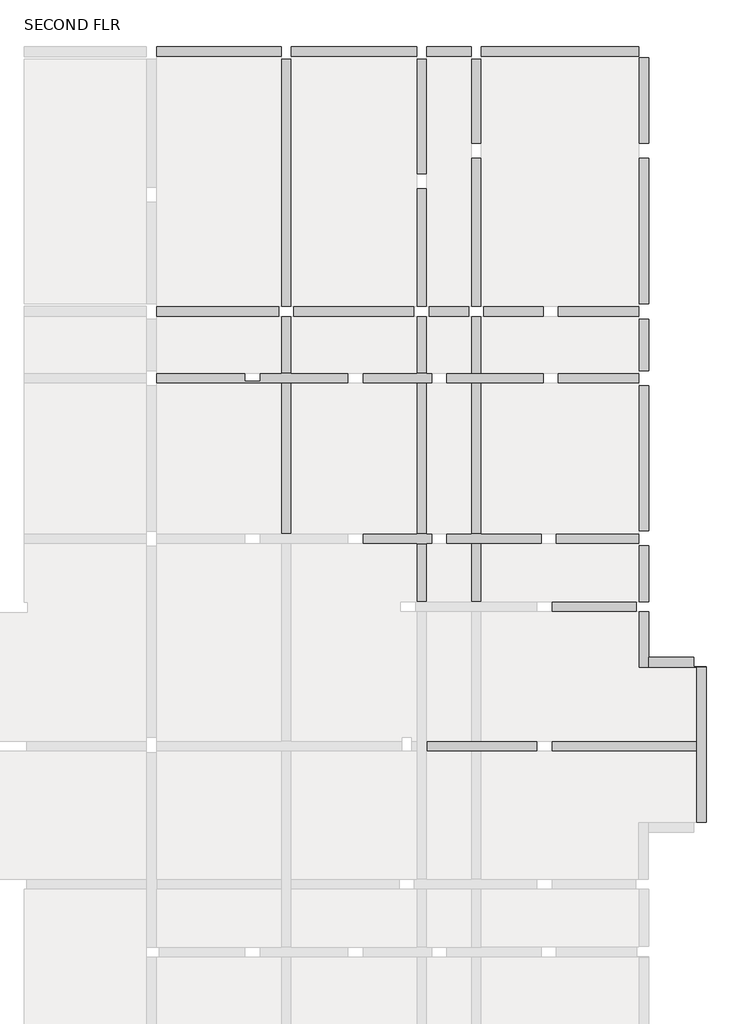
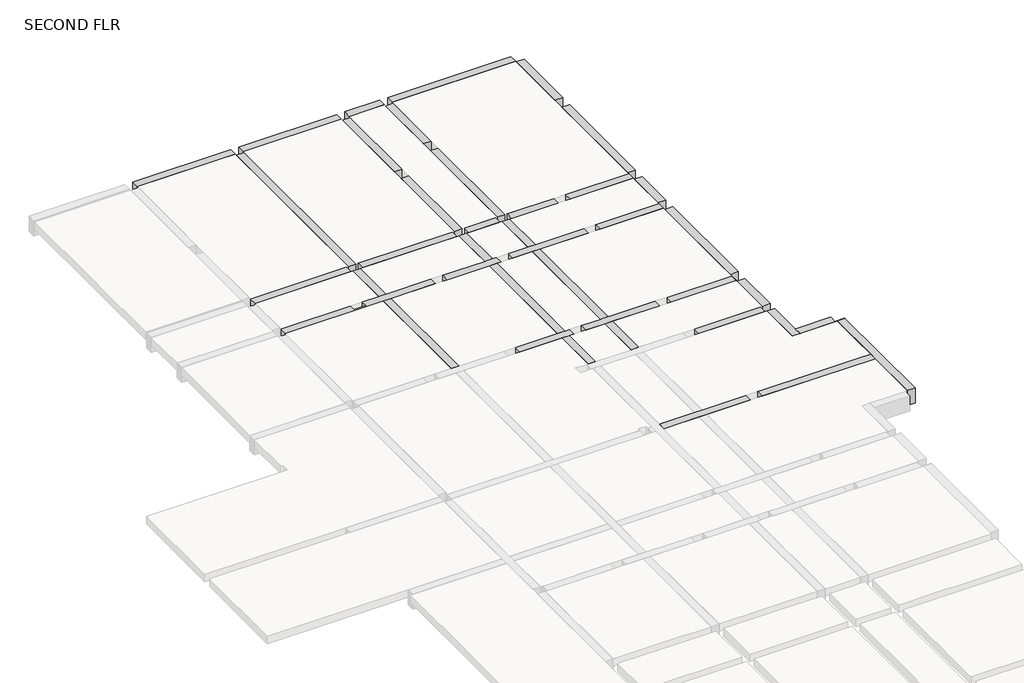
# One storey, part 4 of 4: 40 beams.
"""IFC4 building model written with IfcOpenShell, lengths in millimetres."""

from ifc_helpers import new_model, si_unit, frame, origin, place, context, project, spatial, polyline, outline, extrude, faceted_brep, element, save

model = new_model("IFC4")

# Units and contexts
model_context = context("Model", 3, world=origin())
ifc_project = project(units=[si_unit("LENGTHUNIT", "METRE", prefix="MILLI")], contexts=[model_context])

# Site, building, storey
site = spatial("IfcSite", under=ifc_project)
building = spatial("IfcBuilding", under=site)
storey = spatial("IfcBuildingStorey", under=building, Name="SECOND FLR", Elevation=6048.0)

# Beams
placement = place(None, origin())
element("IfcBeam", 1, ObjectType="M_Concrete-Rectangular Beam : 300 x 600mm", at=placement, inside=storey, context=model_context, shape_type="Brep", body=[
    faceted_brep([(2024.7296816, 21537.8349362, 6048.0), (2024.7296816, 21837.8349362, 6048.0), (-1671.7865686, 21837.8349362, 6048.0), (-1671.7865686, 21537.8349362, 6048.0), (2024.7296816, 21537.8349362, 5448.0), (2024.7296816, 21537.8349362, 5748.0), (-1671.7865686, 21537.8349362, 5748.0), (-1671.7865686, 21537.8349362, 5448.0), (2024.7296816, 21837.8349362, 5448.0), (-1671.7865686, 21837.8349362, 5448.0)], [[[0, 1, 2, 3]], [[4, 5, 0, 3, 6, 7]], [[8, 4, 7, 9]], [[1, 8, 9, 2]], [[2, 9, 7, 6, 3]], [[1, 0, 5, 4, 8]]]),
])
element("IfcBeam", 2, ObjectType="M_Concrete-Rectangular Beam : 300 x 600mm", at=placement, inside=storey, context=model_context, shape_type="Brep", body=[
    faceted_brep([(6032.5248054, 21537.8349362, 6048.0), (6032.5248054, 21837.8349362, 6048.0), (2324.7296816, 21837.8349362, 6048.0), (2324.7296816, 21537.8349362, 6048.0), (6032.5248054, 21537.8349362, 5448.0), (6032.5248054, 21537.8349362, 5748.0), (2324.7296816, 21537.8349362, 5748.0), (2324.7296816, 21537.8349362, 5448.0), (6032.5248054, 21837.8349362, 5448.0), (2324.7296816, 21837.8349362, 5448.0)], [[[0, 1, 2, 3]], [[4, 5, 0, 3, 6, 7]], [[8, 4, 7, 9]], [[1, 8, 9, 2]], [[2, 9, 7, 6, 3]], [[1, 0, 5, 4, 8]]]),
])
element("IfcBeam", 3, ObjectType="M_Concrete-Rectangular Beam : 300 x 600mm", at=placement, inside=storey, context=model_context, shape_type="Brep", body=[
    faceted_brep([(7656.8679014, 21537.8349362, 6048.0), (7656.8679014, 21837.8349362, 6048.0), (6332.5248054, 21837.8349362, 6048.0), (6332.5248054, 21537.8349362, 6048.0), (7656.8679014, 21537.8349362, 5448.0), (7656.8679014, 21537.8349362, 5748.0), (6332.5248054, 21537.8349362, 5748.0), (6332.5248054, 21537.8349362, 5448.0), (7656.8679014, 21837.8349362, 5448.0), (6332.5248054, 21837.8349362, 5448.0)], [[[0, 1, 2, 3]], [[4, 5, 0, 3, 6, 7]], [[8, 4, 7, 9]], [[1, 8, 9, 2]], [[2, 9, 7, 6, 3]], [[1, 0, 5, 4, 8]]]),
])
element("IfcBeam", 4, ObjectType="M_Concrete-Rectangular Beam : 300 x 600mm", at=placement, inside=storey, context=model_context, shape_type="Brep", body=[
    faceted_brep([(7956.8679014, 21837.8349362, 6048.0), (7956.8679014, 21537.8349362, 6048.0), (12619.1163908, 21537.8349362, 6048.0), (12619.1163908, 21837.8349362, 6048.0), (7956.8679014, 21537.8349362, 5748.0), (7956.8679014, 21537.8349362, 5448.0), (12619.1163908, 21537.8349362, 5448.0), (12619.1163908, 21537.8349362, 5748.0), (7956.8679014, 21837.8349362, 5448.0), (12619.1163908, 21837.8349362, 5448.0)], [[[0, 1, 2, 3]], [[1, 4, 5, 6, 7, 2]], [[5, 8, 9, 6]], [[8, 0, 3, 9]], [[0, 8, 5, 4, 1]], [[3, 2, 7, 6, 9]]]),
])
element("IfcBeam", 5, ObjectType="M_Concrete-Rectangular Beam : 300 x 600mm", at=placement, inside=storey, context=model_context, shape_type="Brep", body=[
    faceted_brep([(14319.1163908, 3443.0536525, 6048.0), (14619.1163908, 3443.0536525, 6048.0), (14619.1163908, 3443.0536525, 5448.0), (14319.1163908, 3443.0536525, 5448.0), (14319.1163908, 3435.7536525, 6048.0), (14319.1163908, 1251.1713929, 6048.0), (14319.1163908, 951.1713929, 6048.0), (14319.1163908, -1148.8286071, 6048.0), (14619.1163908, -1148.8286071, 6048.0), (14619.1163908, -1148.8286071, 5448.0), (14319.1163908, -1148.8286071, 5448.0), (14319.1163908, 951.1713929, 5448.0), (14319.1163908, 1251.1713929, 5448.0), (14319.1163908, 3435.7536525, 5448.0), (14319.1163908, -1148.8286071, 5748.0)], [[[0, 1, 2, 3]], [[1, 0, 4, 5, 6, 7, 8]], [[2, 1, 8, 9]], [[3, 2, 9, 10, 11, 12, 13]], [[0, 3, 13, 12, 11, 10, 14, 7, 6, 5, 4]], [[7, 14, 10, 9, 8]]]),
])
element("IfcBeam", 6, ObjectType="M_Concrete-Rectangular Beam : 300 x 600mm", at=placement, inside=storey, context=model_context, shape_type="Brep", body=[
    faceted_brep([(12916.8679014, 5087.6057249, 6048.0), (12616.8679014, 5087.6057249, 6048.0), (12616.8679014, 3435.7536525, 6048.0), (12916.8679014, 3435.7536525, 6048.0), (12916.8679014, 3735.7536525, 6048.0), (12616.8679014, 5087.6057249, 5748.0), (12616.8679014, 5087.6057249, 5448.0), (12616.8679014, 3435.7536525, 5448.0), (12616.8679014, 3435.7536525, 5748.0), (12916.8679014, 5087.6057249, 5448.0), (12916.8679014, 3735.7536525, 5448.0), (12916.8679014, 3435.7536525, 5448.0), (12916.8679014, 3435.7536525, 5748.0)], [[[0, 1, 2, 3, 4]], [[2, 1, 5, 6, 7, 8]], [[6, 9, 10, 11, 7]], [[9, 0, 4, 3, 12, 11, 10]], [[0, 9, 6, 5, 1]], [[3, 2, 8, 7, 11, 12]]]),
])
element("IfcBeam", 7, ObjectType="M_Concrete-Rectangular Beam : 300 x 600mm", at=placement, inside=storey, context=model_context, shape_type="Brep", body=[
    faceted_brep([(12916.8679014, 3735.7536525, 6048.0), (12916.8679014, 3435.7536525, 6048.0), (14319.1163908, 3435.7536525, 6048.0), (14319.1163908, 3443.0536525, 6048.0), (14619.1163908, 3443.0536525, 6048.0), (14619.1163908, 3455.7536525, 6048.0), (14244.1163908, 3455.7536525, 6048.0), (14244.1163908, 3735.7536525, 6048.0), (12916.8679014, 3735.7536525, 5448.0), (14244.1163908, 3735.7536525, 5448.0), (12916.8679014, 3435.7536525, 5448.0), (14244.1163908, 3455.7536525, 5448.0), (14619.1163908, 3455.7536525, 5448.0), (14619.1163908, 3443.0536525, 5448.0), (14319.1163908, 3443.0536525, 5448.0), (14319.1163908, 3435.7536525, 5448.0), (12916.8679014, 3435.7536525, 5748.0), (14319.1163908, 3435.7536525, 5748.0)], [[[0, 1, 2, 3, 4, 5, 6, 7]], [[8, 0, 7, 9]], [[10, 8, 9, 11, 12, 13, 14, 15]], [[2, 1, 16, 10, 15, 17]], [[1, 0, 8, 10, 16]], [[12, 5, 4, 13]], [[7, 6, 11, 9]], [[11, 6, 5, 12]], [[3, 14, 13, 4]], [[14, 3, 2, 17, 15]]]),
])
element("IfcBeam", 8, ObjectType="M_Concrete-Rectangular Beam : 300 x 600mm", at=placement, inside=storey, context=model_context, shape_type="Brep", body=[
    faceted_brep([(12616.8679014, 5387.6057249, 6048.0), (12916.8679014, 5387.6057249, 6048.0), (12916.8679014, 7044.7076276, 6048.0), (12619.1163908, 7044.7076276, 6048.0), (12619.1163908, 7399.7076276, 6048.0), (12616.8679014, 7399.7076276, 6048.0), (12616.8679014, 7099.7076276, 6048.0), (12616.8679014, 7399.7076276, 5448.0), (12616.8679014, 7099.7076276, 5448.0), (12616.8679014, 5387.6057249, 5448.0), (12616.8679014, 5387.6057249, 5748.0), (12616.8679014, 7399.7076276, 5748.0), (12916.8679014, 5387.6057249, 5448.0), (12619.1163908, 7399.7076276, 5448.0), (12619.1163908, 7044.7076276, 5448.0), (12916.8679014, 7044.7076276, 5448.0)], [[[0, 1, 2, 3, 4, 5, 6]], [[7, 8, 9, 10, 0, 6, 5, 11]], [[12, 9, 8, 7, 13, 14, 15]], [[1, 12, 15, 2]], [[1, 0, 10, 9, 12]], [[14, 3, 2, 15]], [[3, 14, 13, 4]], [[5, 4, 13, 7, 11]]]),
])
element("IfcBeam", 9, ObjectType="M_Concrete-Rectangular Beam : 300 x 600mm", at=placement, inside=storey, context=model_context, shape_type="SweptSolid", body=[
    extrude(outline(polyline([(12619.1163908, 11782.4075451), (12919.1163908, 11782.4075451), (12919.1163908, 7494.7076276), (12619.1163908, 7494.7076276), (12619.1163908, 11782.4075451)])), frame((0.0, 0.0, 5448.0), z_axis=(0.0, 0.0, 1.0), x_axis=(1.0, 0.0, 0.0)), (0.0, 0.0, 1.0), 600.0),
])
element("IfcBeam", 10, ObjectType="M_Concrete-Rectangular Beam : 300 x 600mm", at=placement, inside=storey, context=model_context, shape_type="Brep", body=[
    faceted_brep([(12619.1163908, 13762.5179708, 6048.0), (12619.1163908, 12232.4075451, 6048.0), (12919.1163908, 12232.4075451, 6048.0), (12919.1163908, 13762.5179708, 6048.0), (12919.1163908, 12232.4075451, 5448.0), (12919.1163908, 13762.5179708, 5448.0), (12619.1163908, 12232.4075451, 5448.0), (12619.1163908, 13762.5179708, 5448.0), (12619.1163908, 13762.5179708, 5748.0), (12619.1163908, 12232.4075451, 5748.0)], [[[0, 1, 2, 3]], [[3, 2, 4, 5]], [[5, 4, 6, 7]], [[1, 0, 8, 7, 6, 9]], [[0, 3, 5, 7, 8]], [[6, 4, 2, 1, 9]]]),
])
element("IfcBeam", 11, ObjectType="M_Concrete-Rectangular Beam : 300 x 600mm", at=placement, inside=storey, context=model_context, shape_type="Brep", body=[
    faceted_brep([(12619.1163908, 18524.7148651, 6048.0), (12619.1163908, 14212.5179708, 6048.0), (12919.1163908, 14212.5179708, 6048.0), (12919.1163908, 18524.7148651, 6048.0), (12919.1163908, 14212.5179708, 5448.0), (12919.1163908, 18524.7148651, 5448.0), (12619.1163908, 14212.5179708, 5448.0), (12619.1163908, 18524.7148651, 5448.0), (12619.1163908, 18524.7148651, 5748.0), (12619.1163908, 14212.5179708, 5748.0)], [[[0, 1, 2, 3]], [[3, 2, 4, 5]], [[5, 4, 6, 7]], [[1, 0, 8, 7, 6, 9]], [[0, 3, 5, 7, 8]], [[6, 4, 2, 1, 9]]]),
])
element("IfcBeam", 12, ObjectType="M_Concrete-Rectangular Beam : 300 x 600mm", at=placement, inside=storey, context=model_context, shape_type="Brep", body=[
    faceted_brep([(12619.1163908, 21502.8349362, 6048.0), (12619.1163908, 18974.7148651, 6048.0), (12919.1163908, 18974.7148651, 6048.0), (12919.1163908, 21502.8349362, 6048.0), (12919.1163908, 18974.7148651, 5448.0), (12919.1163908, 21502.8349362, 5448.0), (12619.1163908, 18974.7148651, 5448.0), (12619.1163908, 21502.8349362, 5448.0), (12619.1163908, 21502.8349362, 5748.0), (12619.1163908, 18974.7148651, 5748.0)], [[[0, 1, 2, 3]], [[3, 2, 4, 5]], [[5, 4, 6, 7]], [[1, 0, 8, 7, 6, 9]], [[6, 4, 2, 1, 9]], [[0, 3, 5, 7, 8]]]),
])
element("IfcBeam", 13, ObjectType="M_Concrete-Rectangular Beam : 300 x 600mm", at=placement, inside=storey, context=model_context, shape_type="Brep", body=[
    faceted_brep([(2324.7296816, 21462.8349362, 6048.0), (2024.7296816, 21462.8349362, 6048.0), (2024.7296816, 14137.5179708, 6048.0), (2324.7296816, 14137.5179708, 6048.0), (2024.7296816, 21462.8349362, 5748.0), (2024.7296816, 21462.8349362, 5448.0), (2024.7296816, 14137.5179708, 5448.0), (2024.7296816, 14137.5179708, 5748.0), (2324.7296816, 21462.8349362, 5448.0), (2324.7296816, 14137.5179708, 5448.0), (2324.7296816, 14137.5179708, 5748.0), (2324.7296816, 21462.8349362, 5748.0)], [[[0, 1, 2, 3]], [[2, 1, 4, 5, 6, 7]], [[5, 8, 9, 6]], [[0, 3, 10, 9, 8, 11]], [[1, 0, 11, 8, 5, 4]], [[3, 2, 7, 6, 9, 10]]]),
])
element("IfcBeam", 14, ObjectType="M_Concrete-Rectangular Beam : 300 x 600mm", at=placement, inside=storey, context=model_context, shape_type="Brep", body=[
    faceted_brep([(2324.7296816, 13837.5179708, 6048.0), (2024.7296816, 13837.5179708, 6048.0), (2024.7296816, 12157.4075451, 6048.0), (2324.7296816, 12157.4075451, 6048.0), (2024.7296816, 13837.5179708, 5748.0), (2024.7296816, 13837.5179708, 5448.0), (2024.7296816, 12157.4075451, 5448.0), (2024.7296816, 12157.4075451, 5748.0), (2324.7296816, 13837.5179708, 5448.0), (2324.7296816, 12157.4075451, 5448.0), (2324.7296816, 12157.4075451, 5748.0), (2324.7296816, 13837.5179708, 5748.0)], [[[0, 1, 2, 3]], [[2, 1, 4, 5, 6, 7]], [[5, 8, 9, 6]], [[0, 3, 10, 9, 8, 11]], [[1, 0, 11, 8, 5, 4]], [[3, 2, 7, 6, 9, 10]]]),
])
element("IfcBeam", 15, ObjectType="M_Concrete-Rectangular Beam : 300 x 600mm", at=placement, inside=storey, context=model_context, shape_type="Brep", body=[
    faceted_brep([(6332.5248054, 21462.8349362, 6048.0), (6032.5248054, 21462.8349362, 6048.0), (6032.5248054, 18074.7148651, 6048.0), (6332.5248054, 18074.7148651, 6048.0), (6032.5248054, 21462.8349362, 5748.0), (6032.5248054, 21462.8349362, 5448.0), (6032.5248054, 18074.7148651, 5448.0), (6032.5248054, 18074.7148651, 5748.0), (6332.5248054, 21462.8349362, 5448.0), (6332.5248054, 18074.7148651, 5448.0), (6332.5248054, 18074.7148651, 5748.0), (6332.5248054, 21462.8349362, 5748.0)], [[[0, 1, 2, 3]], [[2, 1, 4, 5, 6, 7]], [[5, 8, 9, 6]], [[0, 3, 10, 9, 8, 11]], [[1, 0, 11, 8, 5, 4]], [[3, 2, 7, 6, 9, 10]]]),
])
element("IfcBeam", 16, ObjectType="M_Concrete-Rectangular Beam : 300 x 600mm", at=placement, inside=storey, context=model_context, shape_type="Brep", body=[
    faceted_brep([(6332.5248054, 17624.7148651, 6048.0), (6032.5248054, 17624.7148651, 6048.0), (6032.5248054, 14137.5179708, 6048.0), (6332.5248054, 14137.5179708, 6048.0), (6032.5248054, 17624.7148651, 5748.0), (6032.5248054, 17624.7148651, 5448.0), (6032.5248054, 14137.5179708, 5448.0), (6032.5248054, 14137.5179708, 5748.0), (6332.5248054, 17624.7148651, 5448.0), (6332.5248054, 14137.5179708, 5448.0), (6332.5248054, 14137.5179708, 5748.0), (6332.5248054, 17624.7148651, 5748.0)], [[[0, 1, 2, 3]], [[2, 1, 4, 5, 6, 7]], [[5, 8, 9, 6]], [[0, 3, 10, 9, 8, 11]], [[1, 0, 11, 8, 5, 4]], [[3, 2, 7, 6, 9, 10]]]),
])
element("IfcBeam", 17, ObjectType="M_Concrete-Rectangular Beam : 300 x 600mm", at=placement, inside=storey, context=model_context, shape_type="Brep", body=[
    faceted_brep([(6332.5248054, 13837.5179708, 6048.0), (6032.5248054, 13837.5179708, 6048.0), (6032.5248054, 12157.4075451, 6048.0), (6332.5248054, 12157.4075451, 6048.0), (6032.5248054, 13837.5179708, 5748.0), (6032.5248054, 13837.5179708, 5448.0), (6032.5248054, 12157.4075451, 5448.0), (6032.5248054, 12157.4075451, 5748.0), (6332.5248054, 13837.5179708, 5448.0), (6332.5248054, 12157.4075451, 5448.0), (6332.5248054, 12157.4075451, 5748.0), (6332.5248054, 13837.5179708, 5748.0)], [[[0, 1, 2, 3]], [[2, 1, 4, 5, 6, 7]], [[5, 8, 9, 6]], [[0, 3, 10, 9, 8, 11]], [[1, 0, 11, 8, 5, 4]], [[3, 2, 7, 6, 9, 10]]]),
])
element("IfcBeam", 18, ObjectType="M_Concrete-Rectangular Beam : 300 x 600mm", at=placement, inside=storey, context=model_context, shape_type="Brep", body=[
    faceted_brep([(7956.8679014, 21462.8349362, 6048.0), (7656.8679014, 21462.8349362, 6048.0), (7656.8679014, 18974.7148651, 6048.0), (7956.8679014, 18974.7148651, 6048.0), (7656.8679014, 21462.8349362, 5748.0), (7656.8679014, 21462.8349362, 5448.0), (7656.8679014, 18974.7148651, 5448.0), (7656.8679014, 18974.7148651, 5748.0), (7956.8679014, 21462.8349362, 5448.0), (7956.8679014, 18974.7148651, 5448.0), (7956.8679014, 18974.7148651, 5748.0), (7956.8679014, 21462.8349362, 5748.0)], [[[0, 1, 2, 3]], [[2, 1, 4, 5, 6, 7]], [[5, 8, 9, 6]], [[0, 3, 10, 9, 8, 11]], [[1, 0, 11, 8, 5, 4]], [[3, 2, 7, 6, 9, 10]]]),
])
element("IfcBeam", 19, ObjectType="M_Concrete-Rectangular Beam : 300 x 600mm", at=placement, inside=storey, context=model_context, shape_type="Brep", body=[
    faceted_brep([(7956.8679014, 18524.7148651, 6048.0), (7656.8679014, 18524.7148651, 6048.0), (7656.8679014, 14137.5179708, 6048.0), (7956.8679014, 14137.5179708, 6048.0), (7656.8679014, 18524.7148651, 5748.0), (7656.8679014, 18524.7148651, 5448.0), (7656.8679014, 14137.5179708, 5448.0), (7656.8679014, 14137.5179708, 5748.0), (7956.8679014, 18524.7148651, 5448.0), (7956.8679014, 14137.5179708, 5448.0), (7956.8679014, 14137.5179708, 5748.0), (7956.8679014, 18524.7148651, 5748.0)], [[[0, 1, 2, 3]], [[2, 1, 4, 5, 6, 7]], [[5, 8, 9, 6]], [[0, 3, 10, 9, 8, 11]], [[1, 0, 11, 8, 5, 4]], [[3, 2, 7, 6, 9, 10]]]),
])
element("IfcBeam", 20, ObjectType="M_Concrete-Rectangular Beam : 300 x 600mm", at=placement, inside=storey, context=model_context, shape_type="Brep", body=[
    faceted_brep([(7956.8679014, 13837.5179708, 6048.0), (7656.8679014, 13837.5179708, 6048.0), (7656.8679014, 12157.4075451, 6048.0), (7956.8679014, 12157.4075451, 6048.0), (7656.8679014, 13837.5179708, 5748.0), (7656.8679014, 13837.5179708, 5448.0), (7656.8679014, 12157.4075451, 5448.0), (7656.8679014, 12157.4075451, 5748.0), (7956.8679014, 13837.5179708, 5448.0), (7956.8679014, 12157.4075451, 5448.0), (7956.8679014, 12157.4075451, 5748.0), (7956.8679014, 13837.5179708, 5748.0)], [[[0, 1, 2, 3]], [[2, 1, 4, 5, 6, 7]], [[5, 8, 9, 6]], [[0, 3, 10, 9, 8, 11]], [[1, 0, 11, 8, 5, 4]], [[3, 2, 7, 6, 9, 10]]]),
])
element("IfcBeam", 21, ObjectType="M_Concrete-Rectangular Beam : 300 x 600mm", at=placement, inside=storey, context=model_context, shape_type="Brep", body=[
    faceted_brep([(-1671.7865686, 14137.5179708, 6048.0), (-1671.7865686, 13837.5179708, 6048.0), (1949.7296816, 13837.5179708, 6048.0), (1949.7296816, 14137.5179708, 6048.0), (-1671.7865686, 13837.5179708, 5748.0), (-1671.7865686, 13837.5179708, 5448.0), (1949.7296816, 13837.5179708, 5448.0), (1949.7296816, 13837.5179708, 5748.0), (-1671.7865686, 14137.5179708, 5448.0), (1949.7296816, 14137.5179708, 5448.0), (1949.7296816, 14137.5179708, 5748.0), (-1671.7865686, 14137.5179708, 5748.0)], [[[0, 1, 2, 3]], [[2, 1, 4, 5, 6, 7]], [[5, 8, 9, 6]], [[0, 3, 10, 9, 8, 11]], [[1, 0, 11, 8, 5, 4]], [[3, 2, 7, 6, 9, 10]]]),
])
element("IfcBeam", 22, ObjectType="M_Concrete-Rectangular Beam : 300 x 600mm", at=placement, inside=storey, context=model_context, shape_type="Brep", body=[
    faceted_brep([(2399.7296816, 14137.5179708, 6048.0), (2399.7296816, 13837.5179708, 6048.0), (5957.5248054, 13837.5179708, 6048.0), (5957.5248054, 14137.5179708, 6048.0), (2399.7296816, 13837.5179708, 5748.0), (2399.7296816, 13837.5179708, 5448.0), (5957.5248054, 13837.5179708, 5448.0), (5957.5248054, 13837.5179708, 5748.0), (2399.7296816, 14137.5179708, 5448.0), (5957.5248054, 14137.5179708, 5448.0), (5957.5248054, 14137.5179708, 5748.0), (2399.7296816, 14137.5179708, 5748.0)], [[[0, 1, 2, 3]], [[2, 1, 4, 5, 6, 7]], [[5, 8, 9, 6]], [[0, 3, 10, 9, 8, 11]], [[1, 0, 11, 8, 5, 4]], [[3, 2, 7, 6, 9, 10]]]),
])
element("IfcBeam", 23, ObjectType="M_Concrete-Rectangular Beam : 300 x 600mm", at=placement, inside=storey, context=model_context, shape_type="Brep", body=[
    faceted_brep([(6407.5248054, 14137.5179708, 6048.0), (6407.5248054, 13837.5179708, 6048.0), (7581.8679014, 13837.5179708, 6048.0), (7581.8679014, 14137.5179708, 6048.0), (6407.5248054, 13837.5179708, 5748.0), (6407.5248054, 13837.5179708, 5448.0), (7581.8679014, 13837.5179708, 5448.0), (7581.8679014, 13837.5179708, 5748.0), (6407.5248054, 14137.5179708, 5448.0), (7581.8679014, 14137.5179708, 5448.0), (7581.8679014, 14137.5179708, 5748.0), (6407.5248054, 14137.5179708, 5748.0)], [[[0, 1, 2, 3]], [[2, 1, 4, 5, 6, 7]], [[5, 8, 9, 6]], [[0, 3, 10, 9, 8, 11]], [[1, 0, 11, 8, 5, 4]], [[3, 2, 7, 6, 9, 10]]]),
])
element("IfcBeam", 24, ObjectType="M_Concrete-Rectangular Beam : 300 x 600mm", at=placement, inside=storey, context=model_context, shape_type="Brep", body=[
    faceted_brep([(8031.8679014, 14137.5179708, 6048.0), (8031.8679014, 13837.5179708, 6048.0), (9781.8679014, 13837.5179708, 6048.0), (9781.8679014, 14137.5179708, 6048.0), (8031.8679014, 13837.5179708, 5748.0), (8031.8679014, 13837.5179708, 5448.0), (9781.8679014, 13837.5179708, 5448.0), (9781.8679014, 13837.5179708, 5748.0), (8031.8679014, 14137.5179708, 5448.0), (9781.8679014, 14137.5179708, 5448.0), (9781.8679014, 14137.5179708, 5748.0), (8031.8679014, 14137.5179708, 5748.0)], [[[0, 1, 2, 3]], [[2, 1, 4, 5, 6, 7]], [[5, 8, 9, 6]], [[0, 3, 10, 9, 8, 11]], [[1, 0, 11, 8, 5, 4]], [[3, 2, 7, 6, 9, 10]]]),
])
element("IfcBeam", 25, ObjectType="M_Concrete-Rectangular Beam : 300 x 600mm", at=placement, inside=storey, context=model_context, shape_type="Brep", body=[
    faceted_brep([(10231.8679014, 14137.5179708, 6048.0), (10231.8679014, 13837.5179708, 6048.0), (12619.1163908, 13837.5179708, 6048.0), (12619.1163908, 14137.5179708, 6048.0), (10231.8679014, 13837.5179708, 5748.0), (10231.8679014, 13837.5179708, 5448.0), (12619.1163908, 13837.5179708, 5448.0), (12619.1163908, 13837.5179708, 5748.0), (10231.8679014, 14137.5179708, 5448.0), (12619.1163908, 14137.5179708, 5448.0), (12619.1163908, 14137.5179708, 5748.0), (10231.8679014, 14137.5179708, 5748.0)], [[[0, 1, 2, 3]], [[2, 1, 4, 5, 6, 7]], [[5, 8, 9, 6]], [[0, 3, 10, 9, 8, 11]], [[1, 0, 11, 8, 5, 4]], [[3, 2, 7, 6, 9, 10]]]),
])
element("IfcBeam", 26, ObjectType="M_Concrete-Rectangular Beam : 300 x 600mm", at=placement, inside=storey, context=model_context, shape_type="Brep", body=[
    faceted_brep([(-1671.7865686, 12157.4075451, 6048.0), (-1671.7865686, 11857.4075451, 6048.0), (2024.7296816, 11857.4075451, 6048.0), (2324.7296816, 11857.4075451, 6048.0), (3997.5248054, 11857.4075451, 6048.0), (3997.5248054, 12157.4075451, 6048.0), (2324.7296816, 12157.4075451, 6048.0), (2024.7296816, 12157.4075451, 6048.0), (1399.7296816, 12157.4075451, 6048.0), (1399.7296816, 11917.4075451, 6048.0), (949.7296816, 11917.4075451, 6048.0), (949.7296816, 12157.4075451, 6048.0), (-1671.7865686, 11857.4075451, 5448.0), (2024.7296816, 11857.4075451, 5448.0), (2324.7296816, 11857.4075451, 5448.0), (3997.5248054, 11857.4075451, 5448.0), (3997.5248054, 11857.4075451, 5748.0), (-1671.7865686, 11857.4075451, 5748.0), (-1671.7865686, 12157.4075451, 5448.0), (949.7296816, 12157.4075451, 5448.0), (949.7296816, 11917.4075451, 5448.0), (1399.7296816, 11917.4075451, 5448.0), (1399.7296816, 12157.4075451, 5448.0), (2024.7296816, 12157.4075451, 5448.0), (2324.7296816, 12157.4075451, 5448.0), (3997.5248054, 12157.4075451, 5448.0), (949.7296816, 12157.4075451, 5748.0), (-1671.7865686, 12157.4075451, 5748.0), (3997.5248054, 12157.4075451, 5748.0), (1399.7296816, 12157.4075451, 5748.0)], [[[0, 1, 2, 3, 4, 5, 6, 7, 8, 9, 10, 11]], [[12, 13, 14, 15, 16, 4, 3, 2, 1, 17]], [[12, 18, 19, 20, 21, 22, 23, 24, 25, 15, 14, 13]], [[0, 11, 26, 19, 18, 27]], [[1, 0, 27, 18, 12, 17]], [[5, 4, 16, 15, 25, 28]], [[20, 10, 9, 21]], [[10, 20, 19, 26, 11]], [[21, 9, 8, 29, 22]], [[25, 24, 23, 22, 29, 8, 7, 6, 5, 28]]]),
])
element("IfcBeam", 27, ObjectType="M_Concrete-Rectangular Beam : 300 x 600mm", at=placement, inside=storey, context=model_context, shape_type="Brep", body=[
    faceted_brep([(4447.5248054, 12157.4075451, 6048.0), (4447.5248054, 11857.4075451, 6048.0), (6032.5248054, 11857.4075451, 6048.0), (6332.5248054, 11857.4075451, 6048.0), (6481.8679014, 11857.4075451, 6048.0), (6481.8679014, 12157.4075451, 6048.0), (6332.5248054, 12157.4075451, 6048.0), (6032.5248054, 12157.4075451, 6048.0), (4447.5248054, 11857.4075451, 5448.0), (6032.5248054, 11857.4075451, 5448.0), (6332.5248054, 11857.4075451, 5448.0), (6481.8679014, 11857.4075451, 5448.0), (6481.8679014, 11857.4075451, 5748.0), (4447.5248054, 11857.4075451, 5748.0), (4447.5248054, 12157.4075451, 5448.0), (6032.5248054, 12157.4075451, 5448.0), (6332.5248054, 12157.4075451, 5448.0), (6481.8679014, 12157.4075451, 5448.0), (4447.5248054, 12157.4075451, 5748.0), (6481.8679014, 12157.4075451, 5748.0)], [[[0, 1, 2, 3, 4, 5, 6, 7]], [[8, 9, 10, 11, 12, 4, 3, 2, 1, 13]], [[8, 14, 15, 16, 17, 11, 10, 9]], [[17, 16, 15, 14, 18, 0, 7, 6, 5, 19]], [[1, 0, 18, 14, 8, 13]], [[5, 4, 12, 11, 17, 19]]]),
])
element("IfcBeam", 28, ObjectType="M_Concrete-Rectangular Beam : 300 x 600mm", at=placement, inside=storey, context=model_context, shape_type="Brep", body=[
    faceted_brep([(6931.8679014, 12157.4075451, 6048.0), (6931.8679014, 11857.4075451, 6048.0), (7656.8679014, 11857.4075451, 6048.0), (7956.8679014, 11857.4075451, 6048.0), (9781.8679014, 11857.4075451, 6048.0), (9781.8679014, 12157.4075451, 6048.0), (7956.8679014, 12157.4075451, 6048.0), (7656.8679014, 12157.4075451, 6048.0), (6931.8679014, 11857.4075451, 5448.0), (7656.8679014, 11857.4075451, 5448.0), (7956.8679014, 11857.4075451, 5448.0), (9781.8679014, 11857.4075451, 5448.0), (9781.8679014, 11857.4075451, 5748.0), (6931.8679014, 11857.4075451, 5748.0), (6931.8679014, 12157.4075451, 5448.0), (7656.8679014, 12157.4075451, 5448.0), (7956.8679014, 12157.4075451, 5448.0), (9781.8679014, 12157.4075451, 5448.0), (6931.8679014, 12157.4075451, 5748.0), (9781.8679014, 12157.4075451, 5748.0)], [[[0, 1, 2, 3, 4, 5, 6, 7]], [[8, 9, 10, 11, 12, 4, 3, 2, 1, 13]], [[8, 14, 15, 16, 17, 11, 10, 9]], [[17, 16, 15, 14, 18, 0, 7, 6, 5, 19]], [[1, 0, 18, 14, 8, 13]], [[5, 4, 12, 11, 17, 19]]]),
])
element("IfcBeam", 29, ObjectType="M_Concrete-Rectangular Beam : 300 x 600mm", at=placement, inside=storey, context=model_context, shape_type="Brep", body=[
    faceted_brep([(10231.8679014, 12157.4075451, 6048.0), (10231.8679014, 11857.4075451, 6048.0), (12616.8679014, 11857.4075451, 6048.0), (12619.1163908, 11857.4075451, 6048.0), (12619.1163908, 12157.4075451, 6048.0), (10231.8679014, 11857.4075451, 5448.0), (12619.1163908, 11857.4075451, 5448.0), (10231.8679014, 11857.4075451, 5748.0), (10231.8679014, 12157.4075451, 5448.0), (12619.1163908, 12157.4075451, 5448.0), (12619.1163908, 12157.4075451, 5748.0), (10231.8679014, 12157.4075451, 5748.0)], [[[0, 1, 2, 3, 4]], [[5, 6, 3, 2, 1, 7]], [[5, 8, 9, 6]], [[0, 4, 10, 9, 8, 11]], [[1, 0, 11, 8, 5, 7]], [[4, 3, 6, 9, 10]]]),
])
element("IfcBeam", 30, ObjectType="M_Concrete-Rectangular Beam : 300 x 600mm", at=placement, inside=storey, context=model_context, shape_type="Brep", body=[
    faceted_brep([(4447.5248054, 7399.7076276, 6048.0), (4447.5248054, 7099.7076276, 6048.0), (6032.5248054, 7099.7076276, 6048.0), (6332.5248054, 7099.7076276, 6048.0), (6481.8679014, 7099.7076276, 6048.0), (6481.8679014, 7399.7076276, 6048.0), (6332.5248054, 7399.7076276, 6048.0), (6032.5248054, 7399.7076276, 6048.0), (4447.5248054, 7099.7076276, 5448.0), (6032.5248054, 7099.7076276, 5448.0), (6332.5248054, 7099.7076276, 5448.0), (6481.8679014, 7099.7076276, 5448.0), (6481.8679014, 7099.7076276, 5748.0), (4447.5248054, 7099.7076276, 5748.0), (4447.5248054, 7399.7076276, 5448.0), (6032.5248054, 7399.7076276, 5448.0), (6332.5248054, 7399.7076276, 5448.0), (6481.8679014, 7399.7076276, 5448.0), (4447.5248054, 7399.7076276, 5748.0), (6481.8679014, 7399.7076276, 5748.0)], [[[0, 1, 2, 3, 4, 5, 6, 7]], [[8, 9, 10, 11, 12, 4, 3, 2, 1, 13]], [[8, 14, 15, 16, 17, 11, 10, 9]], [[17, 16, 15, 14, 18, 0, 7, 6, 5, 19]], [[1, 0, 18, 14, 8, 13]], [[5, 4, 12, 11, 17, 19]]]),
])
element("IfcBeam", 31, ObjectType="M_Concrete-Rectangular Beam : 300 x 600mm", at=placement, inside=storey, context=model_context, shape_type="Brep", body=[
    faceted_brep([(6931.8679014, 7399.7076276, 6048.0), (6931.8679014, 7099.7076276, 6048.0), (7656.8679014, 7099.7076276, 6048.0), (7956.8679014, 7099.7076276, 6048.0), (9721.8679014, 7099.7076276, 6048.0), (9721.8679014, 7399.7076276, 6048.0), (7956.8679014, 7399.7076276, 6048.0), (7656.8679014, 7399.7076276, 6048.0), (6931.8679014, 7099.7076276, 5448.0), (7656.8679014, 7099.7076276, 5448.0), (7956.8679014, 7099.7076276, 5448.0), (9721.8679014, 7099.7076276, 5448.0), (9721.8679014, 7099.7076276, 5748.0), (6931.8679014, 7099.7076276, 5748.0), (6931.8679014, 7399.7076276, 5448.0), (7656.8679014, 7399.7076276, 5448.0), (7956.8679014, 7399.7076276, 5448.0), (9721.8679014, 7399.7076276, 5448.0), (6931.8679014, 7399.7076276, 5748.0), (9721.8679014, 7399.7076276, 5748.0)], [[[0, 1, 2, 3, 4, 5, 6, 7]], [[8, 9, 10, 11, 12, 4, 3, 2, 1, 13]], [[8, 14, 15, 16, 17, 11, 10, 9]], [[17, 16, 15, 14, 18, 0, 7, 6, 5, 19]], [[1, 0, 18, 14, 8, 13]], [[5, 4, 12, 11, 17, 19]]]),
])
element("IfcBeam", 32, ObjectType="M_Concrete-Rectangular Beam : 300 x 600mm", at=placement, inside=storey, context=model_context, shape_type="Brep", body=[
    faceted_brep([(10051.8679014, 5387.6057249, 6048.0), (10051.8679014, 5087.6057249, 6048.0), (12541.8679014, 5087.6057249, 6048.0), (12541.8679014, 5387.6057249, 6048.0), (10051.8679014, 5087.6057249, 5748.0), (10051.8679014, 5087.6057249, 5448.0), (12541.8679014, 5087.6057249, 5448.0), (12541.8679014, 5087.6057249, 5748.0), (10051.8679014, 5387.6057249, 5448.0), (12541.8679014, 5387.6057249, 5448.0), (12541.8679014, 5387.6057249, 5748.0), (10051.8679014, 5387.6057249, 5748.0)], [[[0, 1, 2, 3]], [[2, 1, 4, 5, 6, 7]], [[5, 8, 9, 6]], [[0, 3, 10, 9, 8, 11]], [[1, 0, 11, 8, 5, 4]], [[3, 2, 7, 6, 9, 10]]]),
])
element("IfcBeam", 33, ObjectType="M_Concrete-Rectangular Beam : 300 x 600mm", at=placement, inside=storey, context=model_context, shape_type="Brep", body=[
    faceted_brep([(10051.8679014, 1251.1713929, 6048.0), (10051.8679014, 951.1713929, 6048.0), (14319.1163908, 951.1713929, 6048.0), (14319.1163908, 1251.1713929, 6048.0), (10051.8679014, 951.1713929, 5748.0), (10051.8679014, 951.1713929, 5448.0), (14319.1163908, 951.1713929, 5448.0), (14319.1163908, 951.1713929, 5748.0), (10051.8679014, 1251.1713929, 5448.0), (14319.1163908, 1251.1713929, 5448.0), (14319.1163908, 1251.1713929, 5748.0), (10051.8679014, 1251.1713929, 5748.0)], [[[0, 1, 2, 3]], [[2, 1, 4, 5, 6, 7]], [[5, 8, 9, 6]], [[0, 3, 10, 9, 8, 11]], [[1, 0, 11, 8, 5, 4]], [[3, 2, 7, 6, 9, 10]]]),
])
element("IfcBeam", 34, ObjectType="M_Concrete-Rectangular Beam : 300 x 600mm", at=placement, inside=storey, context=model_context, shape_type="Brep", body=[
    faceted_brep([(2324.7296816, 11857.4075451, 6048.0), (2024.7296816, 11857.4075451, 6048.0), (2024.7296816, 7399.7076276, 6048.0), (2324.7296816, 7399.7076276, 6048.0), (2024.7296816, 11857.4075451, 5748.0), (2024.7296816, 11857.4075451, 5448.0), (2024.7296816, 7399.7076276, 5448.0), (2024.7296816, 7399.7076276, 5748.0), (2324.7296816, 11857.4075451, 5448.0), (2324.7296816, 7399.7076276, 5448.0), (2324.7296816, 7399.7076276, 5748.0), (2324.7296816, 11857.4075451, 5748.0)], [[[0, 1, 2, 3]], [[2, 1, 4, 5, 6, 7]], [[5, 8, 9, 6]], [[0, 3, 10, 9, 8, 11]], [[1, 0, 11, 8, 5, 4]], [[3, 2, 7, 6, 9, 10]]]),
])
element("IfcBeam", 35, ObjectType="M_Concrete-Rectangular Beam : 300 x 600mm", at=placement, inside=storey, context=model_context, shape_type="Brep", body=[
    faceted_brep([(6332.5248054, 11857.4075451, 6048.0), (6032.5248054, 11857.4075451, 6048.0), (6032.5248054, 7399.7076276, 6048.0), (6332.5248054, 7399.7076276, 6048.0), (6032.5248054, 11857.4075451, 5748.0), (6032.5248054, 11857.4075451, 5448.0), (6032.5248054, 7399.7076276, 5448.0), (6032.5248054, 7399.7076276, 5748.0), (6332.5248054, 11857.4075451, 5448.0), (6332.5248054, 7399.7076276, 5448.0), (6332.5248054, 7399.7076276, 5748.0), (6332.5248054, 11857.4075451, 5748.0)], [[[0, 1, 2, 3]], [[2, 1, 4, 5, 6, 7]], [[5, 8, 9, 6]], [[0, 3, 10, 9, 8, 11]], [[1, 0, 11, 8, 5, 4]], [[3, 2, 7, 6, 9, 10]]]),
])
element("IfcBeam", 36, ObjectType="M_Concrete-Rectangular Beam : 300 x 600mm", at=placement, inside=storey, context=model_context, shape_type="Brep", body=[
    faceted_brep([(7956.8679014, 11857.4075451, 6048.0), (7656.8679014, 11857.4075451, 6048.0), (7656.8679014, 7399.7076276, 6048.0), (7956.8679014, 7399.7076276, 6048.0), (7656.8679014, 11857.4075451, 5748.0), (7656.8679014, 11857.4075451, 5448.0), (7656.8679014, 7399.7076276, 5448.0), (7656.8679014, 7399.7076276, 5748.0), (7956.8679014, 11857.4075451, 5448.0), (7956.8679014, 7399.7076276, 5448.0), (7956.8679014, 7399.7076276, 5748.0), (7956.8679014, 11857.4075451, 5748.0)], [[[0, 1, 2, 3]], [[2, 1, 4, 5, 6, 7]], [[5, 8, 9, 6]], [[0, 3, 10, 9, 8, 11]], [[1, 0, 11, 8, 5, 4]], [[3, 2, 7, 6, 9, 10]]]),
])
element("IfcBeam", 37, ObjectType="M_Concrete-Rectangular Beam : 300 x 600mm", at=placement, inside=storey, context=model_context, shape_type="Brep", body=[
    faceted_brep([(6332.5248054, 7099.7076276, 6048.0), (6032.5248054, 7099.7076276, 6048.0), (6032.5248054, 5387.6057249, 6048.0), (6332.5248054, 5387.6057249, 6048.0), (6032.5248054, 7099.7076276, 5748.0), (6032.5248054, 7099.7076276, 5448.0), (6032.5248054, 5387.6057249, 5448.0), (6032.5248054, 5387.6057249, 5748.0), (6332.5248054, 7099.7076276, 5448.0), (6332.5248054, 5387.6057249, 5448.0), (6332.5248054, 5387.6057249, 5748.0), (6332.5248054, 7099.7076276, 5748.0)], [[[0, 1, 2, 3]], [[2, 1, 4, 5, 6, 7]], [[5, 8, 9, 6]], [[0, 3, 10, 9, 8, 11]], [[1, 0, 11, 8, 5, 4]], [[3, 2, 7, 6, 9, 10]]]),
])
element("IfcBeam", 38, ObjectType="M_Concrete-Rectangular Beam : 300 x 600mm", at=placement, inside=storey, context=model_context, shape_type="Brep", body=[
    faceted_brep([(7956.8679014, 7099.7076276, 6048.0), (7656.8679014, 7099.7076276, 6048.0), (7656.8679014, 5387.6057249, 6048.0), (7956.8679014, 5387.6057249, 6048.0), (7656.8679014, 7099.7076276, 5748.0), (7656.8679014, 7099.7076276, 5448.0), (7656.8679014, 5387.6057249, 5448.0), (7656.8679014, 5387.6057249, 5748.0), (7956.8679014, 7099.7076276, 5448.0), (7956.8679014, 5387.6057249, 5448.0), (7956.8679014, 5387.6057249, 5748.0), (7956.8679014, 7099.7076276, 5748.0)], [[[0, 1, 2, 3]], [[2, 1, 4, 5, 6, 7]], [[5, 8, 9, 6]], [[0, 3, 10, 9, 8, 11]], [[1, 0, 11, 8, 5, 4]], [[3, 2, 7, 6, 9, 10]]]),
])
element("IfcBeam", 39, ObjectType="M_Concrete-Rectangular Beam : 300 x 600mm", at=placement, inside=storey, context=model_context, shape_type="Brep", body=[
    faceted_brep([(9601.8679014, 951.1713929, 6048.0), (9601.8679014, 1251.1713929, 6048.0), (7956.8679014, 1251.1713929, 6048.0), (7656.8679014, 1251.1713929, 6048.0), (6332.5248054, 1251.1713929, 6048.0), (6332.5248054, 951.1713929, 6048.0), (7656.8679014, 951.1713929, 6048.0), (7956.8679014, 951.1713929, 6048.0), (6332.5248054, 951.1713929, 5448.0), (7656.8679014, 951.1713929, 5448.0), (7956.8679014, 951.1713929, 5448.0), (9601.8679014, 951.1713929, 5448.0), (9601.8679014, 951.1713929, 5748.0), (6332.5248054, 951.1713929, 5748.0), (9601.8679014, 1251.1713929, 5448.0), (6332.5248054, 1251.1713929, 5448.0), (7656.8679014, 1251.1713929, 5448.0), (7956.8679014, 1251.1713929, 5448.0), (6332.5248054, 1251.1713929, 5748.0), (9601.8679014, 1251.1713929, 5748.0)], [[[0, 1, 2, 3, 4, 5, 6, 7]], [[8, 9, 10, 11, 12, 0, 7, 6, 5, 13]], [[14, 11, 10, 9, 8, 15, 16, 17]], [[14, 17, 16, 15, 18, 4, 3, 2, 1, 19]], [[1, 0, 12, 11, 14, 19]], [[5, 4, 18, 15, 8, 13]]]),
])
element("IfcBeam", 40, ObjectType="M_Concrete-Rectangular Beam : 300 x 600mm", at=placement, inside=storey, context=model_context, shape_type="Brep", body=[
    faceted_brep([(10171.8679014, 7399.7076276, 6048.0), (10171.8679014, 7099.7076276, 6048.0), (12616.8679014, 7099.7076276, 6048.0), (12616.8679014, 7399.7076276, 6048.0), (10171.8679014, 7099.7076276, 5748.0), (10171.8679014, 7099.7076276, 5448.0), (12616.8679014, 7099.7076276, 5448.0), (12616.8679014, 7099.7076276, 5748.0), (10171.8679014, 7399.7076276, 5448.0), (12616.8679014, 7399.7076276, 5448.0), (12616.8679014, 7399.7076276, 5748.0), (10171.8679014, 7399.7076276, 5748.0)], [[[0, 1, 2, 3]], [[2, 1, 4, 5, 6, 7]], [[5, 8, 9, 6]], [[0, 3, 10, 9, 8, 11]], [[8, 5, 4, 1, 0, 11]], [[3, 2, 7, 6, 9, 10]]]),
])

save(model, "model.ifc")

# Revit data of these elements
# Type "M_Concrete-Rectangular Beam : 300 x 600mm"
#   Length [instance default] = 1524 mm
#   b = 300 mm
#   h = 600 mm
#   Structural Material [instance default] = Concrete, Cast-in-Place gray
#   Assembly Code = ""
# Elements 1, 2, 3, 4, 5, 6, 7, 8, 9, 10, 11, 12, 13, 14, 15, 16, 17, 18, 19, 20, 21, 22, 23, 24, 25, 26, 27, 28, 29, 30, 31, 32, 33, 40 (IfcBeam, "M_Concrete-Rectangular Beam : 300 x 600mm")
#   Structural Material = Concrete, Cast-in-Place gray
#   Phase Created = New Construction
#   Materials on its faces: "Concrete, Cast-in-Place gray"
# Elements 34, 35, 36, 37, 38, 39 (IfcBeam, "M_Concrete-Rectangular Beam : 300 x 600mm")
#   Phase Created = New Construction
#   Materials on its faces: "Concrete, Cast-in-Place gray"
# Materials
#   "Concrete, Cast-in-Place gray": class "Concrete", colour RGB 192 192 192, transparency 0, Description = "Cast-in-place concrete", Cost = 0
